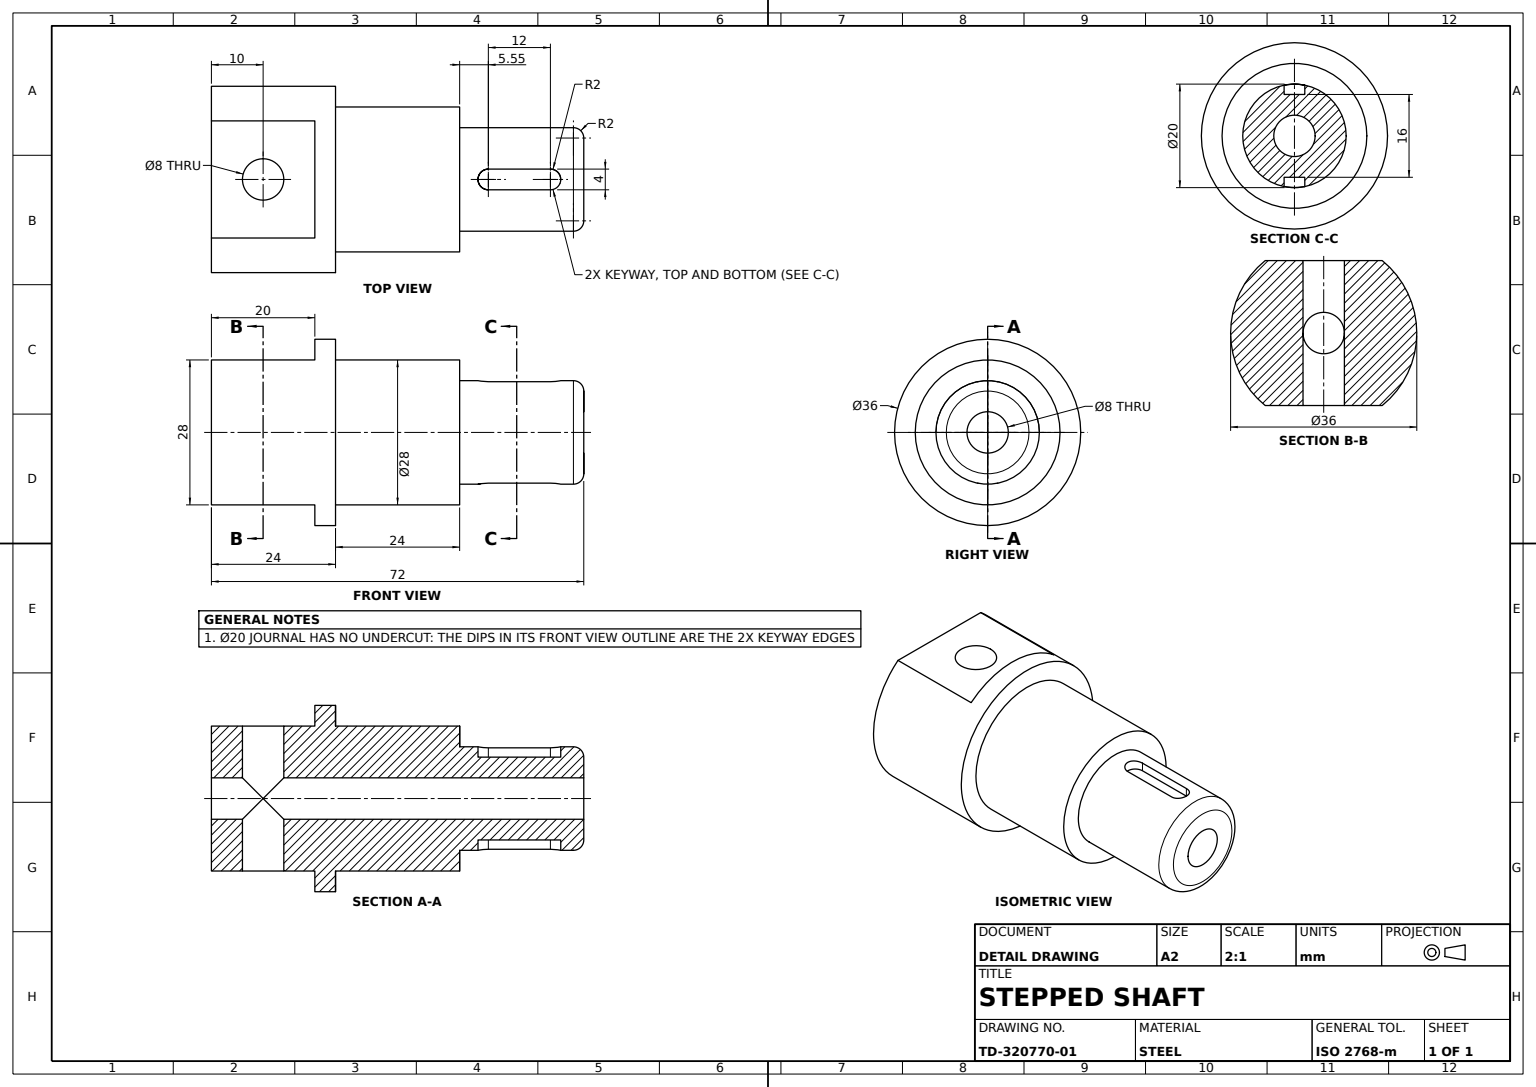
SolidWorks part; units mm, degrees
material "Plain Carbon Steel"
ref_plane "Front Plane" through (0, 0, 0) normal (0, 0, 1) x (1, 0, 0)
ref_plane "Top Plane" through (0, 0, 0) normal (0, 1, 0) x (1, 0, 0)
ref_plane "Right Plane" through (0, 0, 0) normal (1, 0, 0) x (0, 0, -1)
sketch "Shaft Profile Sketch" plane through (0, 0, 0) normal (0, 0, 1) x (1, 0, 0)
  line L0 (0, -40.6316) -> (0, 40.6316) construction
  line L1 (4, 72) -> (4, 0)
  line L2 (4, 0) -> (18, 0)
  line L3 (18, 0) -> (18, 24)
  line L4 (18, 24) -> (14, 24)
  line L5 (14, 24) -> (14, 48)
  line L6 (14, 48) -> (10, 48)
  line L7 (10, 48) -> (10, 72)
  line L8 (10, 72) -> (4, 72)
  point P4 (0, 0)
  dimension "D1" = 4
  dimension "D2" = 10
  dimension "D3" = 4
  dimension "D4" = 4
  dimension "D5" = 24
  dimension "D6" = 24
  dimension "D7" = 24
revolve "Stepped Shaft Body" add sketch "Shaft Profile Sketch" angle 360 about L0
sketch "Base Flat Sketch" plane through (0, 0, 0) normal (0, -1, 0) x (1, 0, 0)
  line L0 (0, 19.9174) -> (0, -19.9174) construction
  line L1 (-14, 11.3137) -> (-14, -11.3137)
  line L2 (14, 11.3137) -> (14, -11.3137)
  arc A0 (14, -11.3137) -> (14, 11.3137) centre (0, 0) ccw
  circle A1 centre (0, 0) radius 18
  arc A2 (-14, 11.3137) -> (-14, -11.3137) centre (0, 0) ccw
  point P6 (0, 0)
  dimension "D1" = 14
  dimension "D2" = 14
  dimension "D3" = 0
extrude "Base Flat" cut sketch "Base Flat Sketch" against normal blind 20
sketch "Cross Hole Sketch" plane through (-14, 0, 0) normal (-1, 0, 0) x (0, 0, 1)
  line L0 (-11.3137, 0) -> (11.3137, 0) construction
  circle A0 centre (0, 10) radius 4
  dimension "D1" = 8
  dimension "D2" = 10
  dimension "D3" = 11.3137
extrude "Cross Hole Ø8" cut sketch "Cross Hole Sketch" against normal blind 30
fillet "Edge Fillet R2" radius 2 1 edges at (0, 72, -10)
ref_plane "Slot Sketch Plane" through (8, 0, 0) normal (1, 0, 0) x (0, 0, -1)
sketch "Slot Sketch" plane through (8, 0, 0) normal (1, 0, 0) x (0, 0, -1)
  line L0 (0, 59.5481) -> (0, 73.9023) construction
  line L1 (-16.0433, 59.5481) -> (31.3847, 59.5481) construction
  line L2 (0, 65.5481) -> (0, 53.5481) construction
  line L3 (2, 65.5481) -> (2, 53.5481)
  line L4 (-2, 65.5481) -> (-2, 53.5481)
  arc A0 (2, 65.5481) -> (-2, 65.5481) centre (0, 65.5481) ccw
  arc A1 (-2, 53.5481) -> (2, 53.5481) centre (0, 53.5481) ccw
  point P7 (0, 59.5481)
  point P13 (0, 51.5481)
  point P14 (0, 67.5481)
  dimension "D1" = 2
  dimension "D2" = 16
  dimension "D3" = 59.5481
extrude "Slot 2x16" cut sketch "Slot Sketch" along normal blind 2
mirror "Slot Mirror" about plane through (0, 0, 0) normal (1, 0, 0) of "Slot 2x16"
